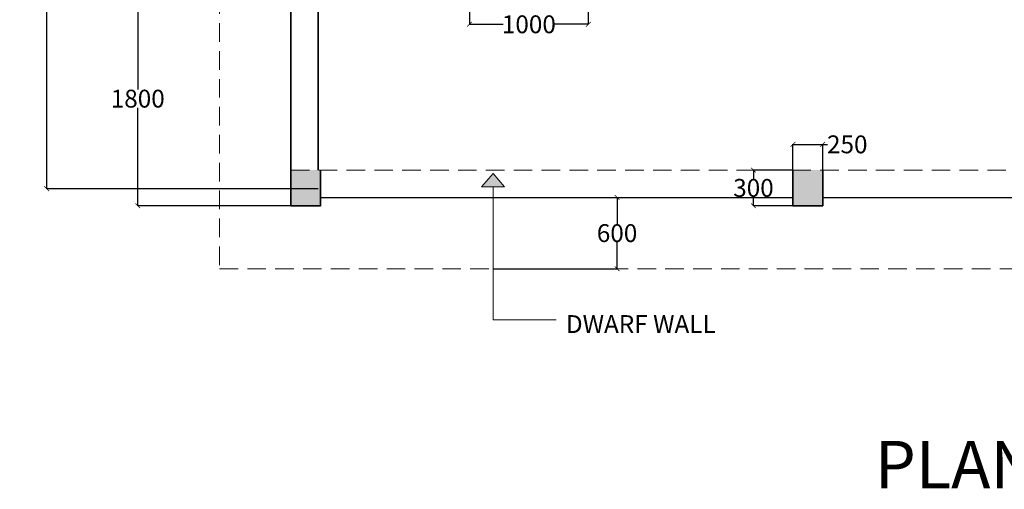
# Model space of a CAD drawing. Units: millimetres. Extents: x 32888 to 53184, y 27889 to 39696.
# Tile 1 of 6: x 32888 to 41170, y 27889 to 31834. Entities that reach past the tile are written whole.
import ezdxf

# ---------------------------------------------------------------- set-up
doc = ezdxf.new("R2010")
doc.units = ezdxf.units.MM
doc.header["$LTSCALE"] = 50
doc.header["$MEASUREMENT"] = 0
doc.linetypes.add('HIDDEN2', pattern=[0.1875, 0.125, -0.0625])
for name, color, linetype, lineweight in [('A-ANNO-DIMS', 2, 'Continuous', 18), ('A-ANNO-SYMB', 7, 'Continuous', 18), ('A-ANNO-SYMB-PATT', 18, 'Continuous', 13), ('A-ANNO-TEXT', 7, 'Continuous', 18), ('A-ANNO-TTLB', 152, 'Continuous', 35), ('A-COLS', 1, 'Continuous', 35), ('A-COLS-PATT', 18, 'Continuous', 18), ('A-ROOF-OVHD', 8, 'HIDDEN2', 18), ('A-WALL', 7, 'Continuous', 35), ('A-WALL-HIDN', 7, 'HIDDEN2', 18), ('A-WALL-LOW', 7, 'Continuous', 25)]:
    doc.layers.add(name, color=color, linetype=linetype, lineweight=lineweight)
doc.styles.get("Standard").update_dxf_attribs({"font": 'arial.ttf'})
doc.dimstyles.get("Standard").update_dxf_attribs({"dimtxt": 150, "dimasz": 40, "dimexe": 0.18, "dimexo": 0.0625, "dimgap": 0.09, "dimtad": 0, "dimtih": 1, "dimtoh": 1, "dimdec": 0, "dimzin": 0, "dimdsep": 46, "dimtxsty": 'Standard', "dimblk": 'ARCHTICK', "dimcen": 0, "dimadec": 0, "dimazin": 0, "dimtfac": 1, "dimtdec": 0, "dimtofl": 0, "dimtmove": 0, "dimatfit": 3, "dimldrblk": 'ARCHTICK', "dimfxl": 1, "dimtolj": 1, "dimtzin": 0, "dimarcsym": 1})

# ---------------------------------------------------------------- blocks, each defined once
blk = doc.blocks.new('_ArchTick')
at = {"color": 0, "linetype": 'ByBlock', "const_width": 0.15}
blk.add_lwpolyline([(-0.5, -0.5), (0.5, 0.5)], dxfattribs=at)
blk = doc.blocks.new('*D5')
at = {"layer": 'A-ANNO-DIMS', "color": 0, "lineweight": -2, "ltscale": 50, "transparency": 16777216}
for p, q in [((39392.6, 30571.1), (39392.6, 30787)), ((39392.6, 30786.8), (39642.6, 30786.8)), ((39642.6, 30571.1), (39642.6, 30787)), ((39642.6, 30786.8), (39682.6, 30786.8))]:
    blk.add_line(p, q, dxfattribs=at)
at = {"layer": 'Defpoints', "color": 0, "ltscale": 50, "transparency": 16777216}
for p in [(39642.6, 30786.8), (39392.6, 30571), (39642.6, 30571)]:
    blk.add_point(p, dxfattribs=at)
at = {"layer": 'A-ANNO-DIMS', "color": 0, "lineweight": -2, "ltscale": 50, "transparency": 16777216, "xscale": 40, "yscale": 40, "zscale": 40, "rotation": 180}
blk.add_blockref('_ArchTick', (39392.6, 30786.8), dxfattribs=at)
at = {"layer": 'A-ANNO-DIMS', "color": 0, "lineweight": -2, "ltscale": 50, "transparency": 16777216, "xscale": 40, "yscale": 40, "zscale": 40}
blk.add_blockref('_ArchTick', (39642.6, 30786.8), dxfattribs=at)
at = {"layer": 'A-ANNO-DIMS', "color": 0, "ltscale": 50, "transparency": 16777216, "insert": (39849.4, 30786.8), "char_height": 150, "attachment_point": 5}
blk.add_mtext('\\A1;250', dxfattribs=at)
blk = doc.blocks.new('*D6')
at = {"layer": 'A-ANNO-DIMS', "color": 0, "lineweight": -2, "ltscale": 50, "transparency": 16777216}
for p, q in [((39392.6, 30571), (39060.1, 30571)), ((39060.3, 30571), (39060.3, 30497.7)), ((39060.3, 30271), (39060.3, 30344.3)), ((39392.6, 30271), (39060.1, 30271))]:
    blk.add_line(p, q, dxfattribs=at)
at = {"layer": 'Defpoints', "color": 0, "ltscale": 50, "transparency": 16777216}
for p in [(39060.3, 30571), (39392.6, 30571), (39392.6, 30271)]:
    blk.add_point(p, dxfattribs=at)
at = {"layer": 'A-ANNO-DIMS', "color": 0, "lineweight": -2, "ltscale": 50, "transparency": 16777216, "xscale": 40, "yscale": 40, "zscale": 40}
for p, rotation in [((39060.3, 30571), 90), ((39060.3, 30271), 270)]:
    blk.add_blockref('_ArchTick', p, dxfattribs=dict(at, rotation=rotation))
at = {"layer": 'A-ANNO-DIMS', "color": 0, "ltscale": 50, "transparency": 16777216, "insert": (39060.3, 30421), "char_height": 150, "attachment_point": 5}
blk.add_mtext('\\A1;300', dxfattribs=at)
blk = doc.blocks.new('*D7')
at = {"layer": 'A-ANNO-DIMS', "color": 0, "lineweight": -2, "ltscale": 50, "transparency": 16777216}
for p, q in [((36870.4, 30341), (37913.2, 30341)), ((37913, 30341), (37913, 30117.7)), ((37913, 29741), (37913, 29964.3)), ((36870.4, 29741), (37913.2, 29741))]:
    blk.add_line(p, q, dxfattribs=at)
at = {"layer": 'Defpoints', "color": 0, "ltscale": 50, "transparency": 16777216}
for p in [(36870.3, 30341), (37913, 30341), (36870.3, 29741)]:
    blk.add_point(p, dxfattribs=at)
at = {"layer": 'A-ANNO-DIMS', "color": 0, "lineweight": -2, "ltscale": 50, "transparency": 16777216, "xscale": 40, "yscale": 40, "zscale": 40}
for p, rotation in [((37913, 30341), 90), ((37913, 29741), 270)]:
    blk.add_blockref('_ArchTick', p, dxfattribs=dict(at, rotation=rotation))
at = {"layer": 'A-ANNO-DIMS', "color": 0, "ltscale": 50, "transparency": 16777216, "insert": (37913, 30041), "char_height": 150, "attachment_point": 5}
blk.add_mtext('\\A1;600', dxfattribs=at)
blk = doc.blocks.new('*D16')
at = {"layer": 'A-ANNO-DIMS', "color": 0, "lineweight": -2, "ltscale": 50, "transparency": 16777216}
for p, q in [((36671.2, 32140.9), (36671.2, 31795.5)), ((37671.2, 32140.9), (37671.2, 31795.5)), ((36671.2, 31795.7), (36954.5, 31795.7)), ((37671.2, 31795.7), (37388, 31795.7))]:
    blk.add_line(p, q, dxfattribs=at)
at = {"layer": 'Defpoints', "color": 0, "ltscale": 50, "transparency": 16777216}
for p in [(36671.2, 32141), (37671.2, 32141), (37671.2, 31795.7)]:
    blk.add_point(p, dxfattribs=at)
at = {"layer": 'A-ANNO-DIMS', "color": 0, "lineweight": -2, "ltscale": 50, "transparency": 16777216, "xscale": 40, "yscale": 40, "zscale": 40, "rotation": 180}
blk.add_blockref('_ArchTick', (36671.2, 31795.7), dxfattribs=at)
at = {"layer": 'A-ANNO-DIMS', "color": 0, "lineweight": -2, "ltscale": 50, "transparency": 16777216, "xscale": 40, "yscale": 40, "zscale": 40}
blk.add_blockref('_ArchTick', (37671.2, 31795.7), dxfattribs=at)
at = {"layer": 'A-ANNO-DIMS', "color": 0, "ltscale": 50, "transparency": 16777216, "insert": (37171.2, 31795.7), "char_height": 150, "attachment_point": 5}
blk.add_mtext('\\A1;1000', dxfattribs=at)
blk = doc.blocks.new('*D22')
at = {"layer": 'A-ANNO-DIMS', "color": 0, "lineweight": -2, "ltscale": 50, "transparency": 16777216}
for p, q in [((35168.9, 32071), (33881.1, 32071)), ((33881.3, 32071), (33881.3, 31247.7)), ((33881.3, 30271), (33881.3, 31094.3)), ((35168.9, 30271), (33881.1, 30271))]:
    blk.add_line(p, q, dxfattribs=at)
at = {"layer": 'Defpoints', "color": 0, "ltscale": 50, "transparency": 16777216}
for p in [(35168.9, 32071), (33881.3, 30271), (35168.9, 30271)]:
    blk.add_point(p, dxfattribs=at)
at = {"layer": 'A-ANNO-DIMS', "color": 0, "lineweight": -2, "ltscale": 50, "transparency": 16777216, "xscale": 40, "yscale": 40, "zscale": 40}
for p, rotation in [((33881.3, 32071), 90), ((33881.3, 30271), 270)]:
    blk.add_blockref('_ArchTick', p, dxfattribs=dict(at, rotation=rotation))
at = {"layer": 'A-ANNO-DIMS', "color": 0, "ltscale": 50, "transparency": 16777216, "insert": (33881.3, 31171), "char_height": 150, "attachment_point": 5}
blk.add_mtext('\\A1;1800', dxfattribs=at)
blk = doc.blocks.new('*D58')
at = {"layer": 'A-ANNO-DIMS', "color": 0, "lineweight": -2, "ltscale": 50, "transparency": 16777216}
for p, q in [((35398.9, 38001), (33115.3, 38001)), ((33115.5, 38001), (33115.5, 34284.2)), ((33115.5, 30414), (33115.5, 34130.8)), ((35398.9, 30414), (33115.3, 30414))]:
    blk.add_line(p, q, dxfattribs=at)
at = {"layer": 'Defpoints', "color": 0, "ltscale": 50, "transparency": 16777216}
for p in [(35398.9, 38001), (33115.5, 30414), (35398.9, 30414)]:
    blk.add_point(p, dxfattribs=at)
at = {"layer": 'A-ANNO-DIMS', "color": 0, "lineweight": -2, "ltscale": 50, "transparency": 16777216, "xscale": 40, "yscale": 40, "zscale": 40}
for p, rotation in [((33115.5, 38001), 90), ((33115.5, 30414), 270)]:
    blk.add_blockref('_ArchTick', p, dxfattribs=dict(at, rotation=rotation))
at = {"layer": 'A-ANNO-DIMS', "color": 0, "ltscale": 50, "transparency": 16777216, "insert": (33115.5, 34207.5), "char_height": 150, "attachment_point": 5}
blk.add_mtext('\\A1;7587', dxfattribs=at)
blk = doc.blocks.new('COLUMN-VERANDAH-250x300')
blk.add_lwpolyline([(0, 300), (0, 0), (250, 0), (250, 300)])

msp = doc.modelspace()

# ---------------------------------------------------------------- hatches: boundary and pattern name
at = {"layer": 'A-ANNO-SYMB-PATT', "ltscale": 50}
h = msp.add_hatch(color=256, dxfattribs=at)
h.dxf.hatch_style = 1
h.paths.add_polyline_path([(36870.29, 30540.94), (36772.99, 30430.6), (36870.29, 30430.6), (36967.6, 30430.6)])
h.paths.add_polyline_path([(48072.03, 30571.01), (47974.72, 30460.67), (48072.03, 30460.67), (48169.34, 30460.67)])
h.paths.add_polyline_path([(51769.69, 35712.9), (51769.69, 35665.99), (51769.69, 35619.08), (51826.03, 35665.99)])
at = {"layer": 'A-COLS-PATT', "ltscale": 50}
h = msp.add_hatch(color=256, dxfattribs=at)
h.dxf.hatch_style = 1
h.paths.add_polyline_path([(35398.95, 38071.01), (35168.95, 38071.01), (35168.95, 37771.01), (35398.95, 37771.01)])
h.paths.add_polyline_path([(39628.95, 38071.01), (39398.95, 38071.01), (39398.95, 37771.01), (39628.95, 37771.01)])
h.paths.add_polyline_path([(43903.95, 38071.01), (43673.95, 38071.01), (43673.95, 37771.01), (43903.95, 37771.01)])
h.paths.add_polyline_path([(47658.95, 38071.01), (47428.95, 38071.01), (47428.95, 37771.01), (47658.95, 37771.01)])
h.paths.add_polyline_path([(50888.95, 38071.01), (50658.95, 38071.01), (50658.95, 37771.01), (50888.95, 37771.01)])
h.paths.add_polyline_path([(50888.95, 35221.01), (50658.95, 35221.01), (50658.95, 34921.01), (50888.95, 34921.01)])
h.paths.add_polyline_path([(47658.95, 35221.01), (47428.95, 35221.01), (47428.95, 34921.01), (47658.95, 34921.01)])
h.paths.add_polyline_path([(39628.95, 35071.01), (39628.95, 35221.01), (39398.95, 35221.01), (39398.95, 34921.01), (39628.95, 34921.01)])
h.paths.add_polyline_path([(35398.95, 35221.01), (35168.95, 35221.01), (35168.95, 34921.01), (35398.95, 34921.01)])
h.paths.add_polyline_path([(35398.95, 32371.01), (35168.95, 32371.01), (35168.95, 32071.01), (35398.95, 32071.01)])
h.paths.add_polyline_path([(35418.95, 30571.01), (35168.95, 30571.01), (35168.95, 30271.01), (35418.95, 30271.01)])
h.paths.add_polyline_path([(39642.61, 30571.01), (39392.61, 30571.01), (39392.61, 30271.01), (39642.61, 30271.01)])
h.paths.add_polyline_path([(39628.95, 32371.01), (39398.95, 32371.01), (39398.95, 32071.01), (39628.95, 32071.01)])
h.paths.add_polyline_path([(43903.95, 32371.01), (43673.95, 32371.01), (43673.95, 32071.01), (43903.95, 32071.01)])
h.paths.add_polyline_path([(43903.95, 30571.01), (43653.95, 30571.01), (43653.95, 30271.01), (43903.95, 30271.01)])
h.paths.add_polyline_path([(47658.95, 32441.01), (47428.95, 32441.01), (47428.95, 32141.01), (47658.95, 32141.01)])
h.paths.add_polyline_path([(50888.95, 32414.45), (50658.95, 32414.45), (50658.95, 32114.45), (50888.95, 32114.45)])
h.paths.add_polyline_path([(50888.95, 30571.01), (50638.95, 30571.01), (50638.95, 30271.01), (50888.95, 30271.01)])
h.paths.add_polyline_path([(47678.95, 30571.01), (47428.95, 30571.01), (47428.95, 30341.01), (47678.95, 30341.01)])
h.paths.add_polyline_path([(47678.95, 30341.01), (47428.95, 30341.01), (47428.95, 30271.01), (47678.95, 30271.01)])

# ---------------------------------------------------------------- linework, layer by layer
at = {"layer": 'A-ANNO-SYMB', "ltscale": 50}
for p, q in [((36870.29, 30540.94), (36772.99, 30430.6)), ((36870.29, 30540.94), (36967.6, 30430.6)), ((36772.99, 30430.6), (36870.29, 30430.6)), ((36870.29, 29313.12), (36870.29, 30430.6)), ((36967.6, 30430.6), (36870.29, 30430.6)), ((36870.29, 29313.12), (37400.73, 29313.12))]:
    msp.add_line(p, q, dxfattribs=at)
at = {"layer": 'A-COLS'}
msp.add_lwpolyline([(35168.95, 30271.01), (35418.95, 30271.01), (35418.95, 30571.01)], dxfattribs=at)
at = {"layer": 'A-ROOF-OVHD', "ltscale": 25}
for p, q in [((34568.95, 38601.01), (34568.95, 29741.01)), ((34568.95, 29741.01), (51488.95, 29741.01))]:
    msp.add_line(p, q, dxfattribs=at)
at = {"layer": 'A-WALL'}
for p, q in [((35168.95, 38736.01), (35168.95, 30271.01)), ((35398.95, 38071.01), (35398.95, 30571.01))]:
    msp.add_line(p, q, dxfattribs=at)
at = {"layer": 'A-WALL-HIDN', "ltscale": 25}
msp.add_line((35168.95, 30571.01), (50888.95, 30571.01), dxfattribs=at)
at = {"layer": 'A-WALL-LOW'}
for p, q in [((35418.95, 30341.01), (39392.61, 30341.01)), ((39642.61, 30341.01), (43653.95, 30341.01))]:
    msp.add_line(p, q, dxfattribs=at)

# ---------------------------------------------------------------- block references
at = {"layer": 'A-COLS'}
msp.add_blockref('COLUMN-VERANDAH-250x300', (39392.62, 30271.01), dxfattribs=at)

# ---------------------------------------------------------------- texts
at = {"layer": 'A-ANNO-TEXT', "ltscale": 50, "insert": (37482.85, 29351.7), "char_height": 150, "attachment_point": 1}
msp.add_mtext_dynamic_manual_height_columns('DWARF WALL', width=1699.3106, gutter_width=1, heights=[0], dxfattribs=at)
at = {"layer": 'A-ANNO-TTLB', "ltscale": 50, "insert": (40080.77, 28295.74), "char_height": 400, "attachment_point": 1}
msp.add_mtext_dynamic_manual_height_columns('PLAN OF A DORMITORY', width=8577.7498, gutter_width=1, heights=[0], dxfattribs=at)

# ---------------------------------------------------------------- dimensions: what is measured, and where the dimension line sits
at = {"layer": 'A-ANNO-DIMS', "ltscale": 50}
for p1, p2, distance, picture, middle in [((35398.95, 38001.01), (35398.95, 30414.01), -2283.42, '*D58', (33115.53, 34207.51)), ((36671.2, 32141.01), (37671.2, 32141.01), -345.35, '*D16', (37171.2, 31795.66)), ((35168.95, 32071.01), (35168.95, 30271.01), -1287.67, '*D22', (33881.28, 31171.01)), ((39392.61, 30571.01), (39642.61, 30571.01), 215.77, '*D5', (39849.43, 30786.78)), ((39392.61, 30271.01), (39392.61, 30571.01), 332.31, '*D6', (39060.31, 30421.01)), ((36870.29, 29741.01), (36870.29, 30341.01), -1042.75, '*D7', (37913.04, 30041.01))]:
    dim = msp.add_aligned_dim(p1=p1, p2=p2, distance=distance, dimstyle='Standard', override={"dimclrd": 0, "dimclre": 0, "dimclrt": 0}, dxfattribs=at)
    dim.commit()
    dim.dimension.update_dxf_attribs({"geometry": picture, "text_midpoint": middle})

doc.saveas('drawing.dxf')
